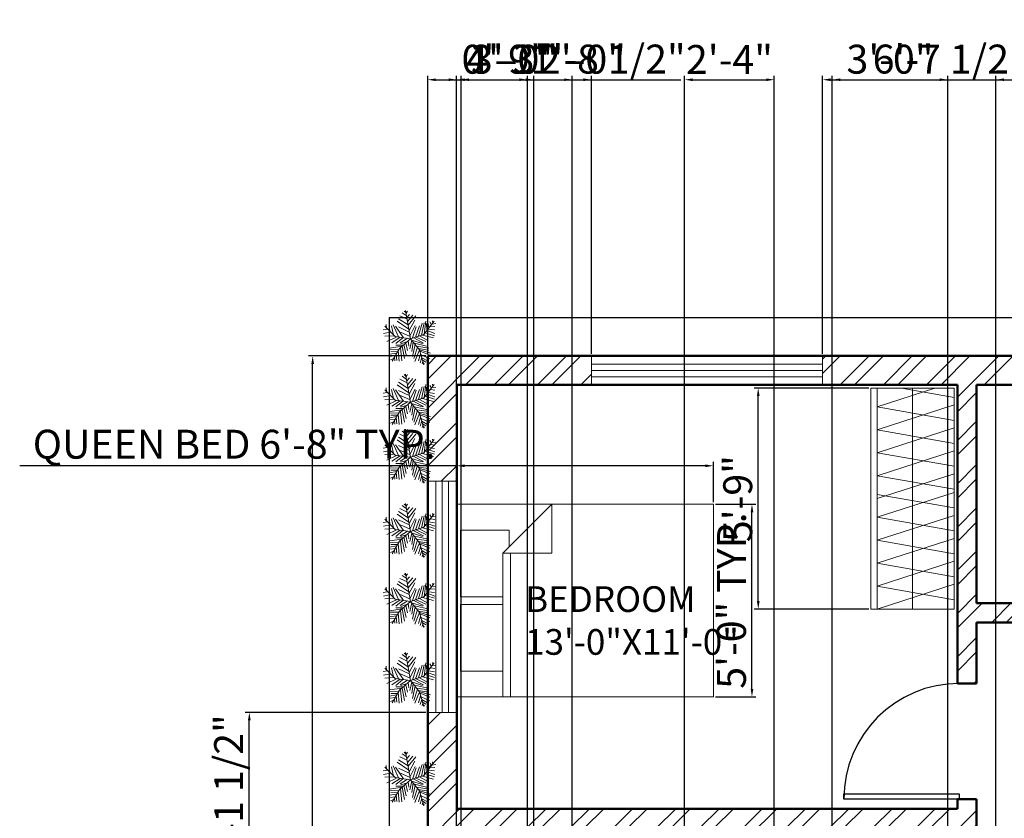
# Model space of a CAD drawing. Units: inches. Extents: x 176 to 806, y 915 to 1663.
# Tile 3 of 5: x 176 to 482, y 1414 to 1663. Entities that reach past the tile are written whole.
import ezdxf

# ---------------------------------------------------------------- set-up
doc = ezdxf.new("R2010")
doc.units = ezdxf.units.IN
for name, color, linetype, lineweight in [('A-ANNO-DIMS', 2, 'Continuous', 18), ('A-AREA-IDEN', 7, 'Continuous', 18), ('A-DOOR', 4, 'Continuous', 25), ('A-FLOR-CASE', 8, 'Continuous', 18), ('A-FURN', 8, 'Continuous', 18), ('A-WALL', 7, 'Continuous', 50), ('A-WALL-PATT', 252, 'Continuous', 13), ('C-PROP', 8, 'Continuous', 25), ('L-PLNT', 3, 'Continuous', 13)]:
    doc.layers.add(name, color=color, linetype=linetype, lineweight=lineweight)
doc.layers.add('A-GLAZ', color=244, linetype='Continuous', lineweight=18, true_color=0x991b1e)
doc.styles.get("Standard").update_dxf_attribs({"font": 'arial.ttf'})
doc.dimstyles.new('ISO-25', dxfattribs={"dimtxt": 9, "dimasz": 2.5, "dimexe": 1.25, "dimexo": 0.625, "dimtad": 1, "dimlunit": 3, "dimtxsty": 'Standard', "dimcen": 2.5, "dimadec": 0, "dimazin": 0, "dimtfac": 1, "dimtmove": 0, "dimatfit": 3, "dimfxl": 1, "dimarcsym": 0})

# ---------------------------------------------------------------- blocks, each defined once
blk = doc.blocks.new('*U4')
for p, q in [((-40, 0), (-40, 6)), ((0, 0), (0, 6))]:
    blk.add_line(p, q)
blk.add_lwpolyline([(0, 0), (0, -40), (-1.75, -40), (-1.75, 0)], close=True)
blk.add_arc((0, 0), 40, 180, 270)
blk = doc.blocks.new('*D10')
at = {"layer": 'A-ANNO-DIMS', "color": 0, "lineweight": -2, "transparency": 16777216}
for p, q in [((302.08, 1558.21), (265.58, 1558.21)), ((266.83, 1052.71), (266.83, 1555.71)), ((302.08, 1050.21), (265.58, 1050.21))]:
    blk.add_line(p, q, dxfattribs=at)
at = {"layer": 'A-ANNO-DIMS', "color": 0, "transparency": 16777216}
for points in [[(266.42, 1555.71), (267.25, 1555.71), (266.83, 1558.21)], [(266.42, 1052.71), (267.25, 1052.71), (266.83, 1050.21)]]:
    blk.add_solid(points, dxfattribs=at)
at = {"layer": 'Defpoints', "color": 0, "transparency": 16777216}
for p in [(266.83, 1558.21), (302.7, 1558.21), (302.7, 1050.21)]:
    blk.add_point(p, dxfattribs=at)
at = {"layer": 'A-ANNO-DIMS', "color": 0, "transparency": 16777216, "insert": (261.69, 1304.21), "char_height": 9, "attachment_point": 5, "rotation": 90}
blk.add_mtext('42\'-4"', dxfattribs=at)
blk = doc.blocks.new('Bed - Queen')
for p, q in [((0, -80.00003), (0, 0)), ((0, 0), (59.99999, 0)), ((59.99999, 0), (59.99999, -80.00003)), ((7.99999, -1.2), (28.79998, -1.2)), ((7.99999, -14.4), (7.99999, -1.2)), ((28.79998, -1.2), (28.79998, -14.4)), ((31.19999, -1.2), (51.99999, -1.2)), ((31.19999, -14.4), (31.19999, -1.2)), ((51.99999, -1.2), (51.99999, -16.4)), ((0, -14.4), (44.8, -14.4)), ((59.99999, -29.6), (44.8, -14.4)), ((44.8, -14.4), (44.8, -29.6)), ((44.8, -16.8), (0, -16.8)), ((51.99999, -16.4), (46.79936, -16.4)), ((44.8, -29.6), (59.99999, -29.6)), ((59.99999, -80.00003), (0, -80.00003))]:
    blk.add_line(p, q)
blk = doc.blocks.new('*U8')
for p, q in [((-5.114, 28.097), (-24.676, 40.636)), ((-7.288, 39.707), (-21.778, 46.673)), ((-8.737, 47.138), (-17.069, 52.711)), ((-10.186, 53.64), (-13.084, 55.962)), ((0, 0), (-10.5, 57)), ((-9.099, 51.782), (-6.563, 55.962)), ((-7.65, 43.423), (-2.578, 49.46)), ((-5.839, 35.992), (4.667, 48.067)), ((-5.114, 27.632), (10.463, 46.673)), ((-31.5, 4.5), (-52.5, 25.5)), ((-48.585, 21.131), (-49.309, 29.026)), ((-43.513, 28.561), (-42.427, 15.558)), ((-38.442, 26.239), (-34.819, 7.663)), ((-35.544, 28.097), (-24.314, 3.947)), ((-14.533, 2.09), (-30.834, 25.31)), ((-3.665, 19.273), (-27.574, 35.527)), ((-24.314, 23.917), (-2.941, 13.7)), ((-2.941, 16.486), (8.652, 37.85)), ((-1.129, 6.734), (9.014, 26.704)), ((3.942, 1.625), (11.187, 24.381)), ((10.101, 3.483), (17.708, 26.239)), ((16.259, 5.805), (23.142, 31.348)), ((22.055, 7.198), (27.489, 32.277)), ((27, 9), (48, 36)), ((27.127, 9.056), (31.112, 35.992)), ((31.836, 30.883), (32.561, 16.486)), ((35.096, 32.741), (37.27, 22.524)), ((38.719, 34.134), (41.979, 28.561)), ((40.53, 25.775), (48.862, 24.846)), ((43.791, 29.954), (51.036, 30.883)), ((44.153, 36.456), (45.239, 32.741)), ((-47.498, 19.737), (-55.83, 18.344)), ((-40.615, 13.7), (-55.105, 10.913)), ((-33.37, 6.269), (-52.207, 5.34)), ((-28.299, 3.483), (-47.86, -5.805)), ((-21.416, 3.018), (-38.079, -8.128)), ((0, 0), (-31.5, 4.5)), ((-15.982, 2.09), (-30.11, -9.521)), ((0, 0), (-22.5, -19.5)), ((-6.563, 1.161), (-21.416, -8.128)), ((-20.691, 13.7), (-1.129, 4.876)), ((0, 0), (27, 9)), ((0, 0), (18, -22.5)), ((6.478, 1.625), (26.04, -8.592)), ((11.187, 3.483), (30.749, -5.805)), ((18.07, 5.805), (35.096, -3.483)), ((24.229, 7.663), (46.688, 1.625)), ((29.662, 12.307), (48.137, 6.269)), ((33.285, 16.486), (48.862, 10.913)), ((36.183, 19.737), (48.137, 17.88)), ((-17.431, -15.094), (-42.789, -18.809)), ((-22.5, -19.5), (-37.5, -45)), ((-15.257, -12.772), (-30.11, -12.772)), ((-20.691, -18.345), (-17.793, -44.352)), ((-6.563, -5.805), (-19.967, -9.985)), ((-17.069, -15.094), (-12.721, -40.172)), ((-13.446, -11.378), (-8.737, -32.741)), ((-9.461, -8.592), (-6.201, -23.453)), ((-4.752, -3.483), (-3.665, -14.629)), ((2.493, -3.019), (-1.491, -20.202)), ((1.769, -2.555), (24.229, -9.521)), ((5.029, -6.27), (2.131, -25.775)), ((9.014, -11.378), (3.58, -35.992)), ((14.085, -16.951), (6.478, -40.172)), ((7.565, -9.056), (32.198, -14.629)), ((12.274, -15.094), (36.907, -18.809)), ((16.259, -19.738), (36.183, -22.989)), ((-28.299, -29.026), (-42.789, -31.348)), ((-24.314, -21.596), (-42.427, -22.06)), ((-30.834, -34.135), (-42.427, -35.528)), ((-34.457, -39.708), (-40.978, -42.494)), ((-26.849, -26.24), (-40.253, -25.775)), ((-32.646, -36.921), (-31.921, -44.352)), ((-29.023, -30.884), (-27.936, -43.887)), ((-25.038, -23.918), (-22.865, -45.281)), ((18.07, -22.524), (8.289, -45.745)), ((20.244, -30.419), (15.897, -44.816)), ((18, -22.5), (27, -52.5)), ((18.433, -22.524), (40.53, -29.026)), ((19.157, -25.311), (38.719, -33.206)), ((22.78, -37.85), (19.519, -48.532)), ((21.331, -32.741), (39.081, -40.636)), ((22.78, -38.314), (34.372, -44.816)), ((24.591, -45.745), (23.142, -50.854)), ((24.591, -43.423), (30.749, -47.603)), ((26.764, -49.925), (28.213, -50.854))]:
    blk.add_line(p, q)
blk = doc.blocks.new('WIN-GLAZING-72IN')
for p, q in [((0, 2), (72, 2)), ((0, 0), (72, 0)), ((0, -2), (72, -2))]:
    blk.add_line(p, q)
blk = doc.blocks.new('WARDROBE-HANGER')
for p, q in [((0, 0), (24, 7.76)), ((24, -4.24), (0, 0))]:
    blk.add_line(p, q)
blk = doc.blocks.new('*D28')
at = {"layer": 'A-ANNO-DIMS', "color": 0, "lineweight": -2, "transparency": 16777216}
for p, q in [((311.7, 1512.63), (311.7, 1525.26)), ((391.7, 1512.63), (391.7, 1525.26)), ((311.7, 1524.01), (175.56, 1524.01)), ((389.2, 1524.01), (314.2, 1524.01))]:
    blk.add_line(p, q, dxfattribs=at)
at = {"layer": 'A-ANNO-DIMS', "color": 0, "transparency": 16777216}
for points in [[(314.2, 1524.42), (314.2, 1523.59), (311.7, 1524.01)], [(389.2, 1524.42), (389.2, 1523.59), (391.7, 1524.01)]]:
    blk.add_solid(points, dxfattribs=at)
at = {"layer": 'Defpoints', "color": 0, "transparency": 16777216}
for p in [(311.7, 1524.01), (311.7, 1512.01), (391.7, 1512.01)]:
    blk.add_point(p, dxfattribs=at)
at = {"layer": 'A-ANNO-DIMS', "color": 0, "transparency": 16777216, "insert": (242.38, 1529.56), "char_height": 9, "attachment_point": 5}
blk.add_mtext('QUEEN BED 6\'-8" TYP.', dxfattribs=at)
blk = doc.blocks.new('*D29')
at = {"layer": 'A-ANNO-DIMS', "color": 0, "lineweight": -2, "transparency": 16777216}
for p, q in [((392.33, 1512.01), (404.95, 1512.01)), ((403.7, 1454.51), (403.7, 1509.51)), ((392.33, 1452.01), (404.95, 1452.01))]:
    blk.add_line(p, q, dxfattribs=at)
at = {"layer": 'A-ANNO-DIMS', "color": 0, "transparency": 16777216}
for points in [[(403.29, 1509.51), (404.12, 1509.51), (403.7, 1512.01)], [(403.29, 1454.51), (404.12, 1454.51), (403.7, 1452.01)]]:
    blk.add_solid(points, dxfattribs=at)
at = {"layer": 'Defpoints', "color": 0, "transparency": 16777216}
for p in [(391.7, 1512.01), (403.7, 1512.01), (391.7, 1452.01)]:
    blk.add_point(p, dxfattribs=at)
at = {"layer": 'A-ANNO-DIMS', "color": 0, "transparency": 16777216, "insert": (398.48, 1482.01), "char_height": 9, "attachment_point": 5, "rotation": 90}
blk.add_mtext('5\'-0" TYP.', dxfattribs=at)
blk = doc.blocks.new('*D40')
at = {"layer": 'A-ANNO-DIMS', "color": 0, "lineweight": -2, "transparency": 16777216}
for p, q in [((302.7, 1558.83), (302.7, 1645.51)), ((305.2, 1644.26), (351.2, 1644.26)), ((353.7, 1558.83), (353.7, 1645.51))]:
    blk.add_line(p, q, dxfattribs=at)
at = {"layer": 'A-ANNO-DIMS', "color": 0, "transparency": 16777216}
for points in [[(305.2, 1644.67), (305.2, 1643.84), (302.7, 1644.26)], [(351.2, 1644.67), (351.2, 1643.84), (353.7, 1644.26)]]:
    blk.add_solid(points, dxfattribs=at)
at = {"layer": 'Defpoints', "color": 0, "transparency": 16777216}
for p in [(353.7, 1644.26), (302.7, 1558.21), (353.7, 1558.21)]:
    blk.add_point(p, dxfattribs=at)
at = {"layer": 'A-ANNO-DIMS', "color": 0, "transparency": 16777216, "insert": (328.2, 1649.48), "char_height": 9, "attachment_point": 5}
blk.add_mtext('4\'-3"', dxfattribs=at)
blk = doc.blocks.new('*D41')
at = {"layer": 'A-ANNO-DIMS', "color": 0, "lineweight": -2, "transparency": 16777216}
for p, q in [((425.7, 1558.83), (425.7, 1645.51)), ((428.2, 1644.26), (502.7, 1644.26)), ((505.2, 1558.83), (505.2, 1645.51))]:
    blk.add_line(p, q, dxfattribs=at)
at = {"layer": 'A-ANNO-DIMS', "color": 0, "transparency": 16777216}
for points in [[(428.2, 1644.67), (428.2, 1643.84), (425.7, 1644.26)], [(502.7, 1644.67), (502.7, 1643.84), (505.2, 1644.26)]]:
    blk.add_solid(points, dxfattribs=at)
at = {"layer": 'Defpoints', "color": 0, "transparency": 16777216}
for p in [(505.2, 1644.26), (425.7, 1558.21), (505.2, 1558.21)]:
    blk.add_point(p, dxfattribs=at)
at = {"layer": 'A-ANNO-DIMS', "color": 0, "transparency": 16777216, "insert": (465.45, 1649.53), "char_height": 9, "attachment_point": 5}
blk.add_mtext('6\'-7 1/2"', dxfattribs=at)
blk = doc.blocks.new('*D48')
at = {"layer": 'A-ANNO-DIMS', "color": 0, "lineweight": -2, "transparency": 16777216}
for p, q in [((302.08, 1447.21), (245.85, 1447.21)), ((247.1, 1400.21), (247.1, 1444.71)), ((302.08, 1397.71), (245.85, 1397.71))]:
    blk.add_line(p, q, dxfattribs=at)
at = {"layer": 'A-ANNO-DIMS', "color": 0, "transparency": 16777216}
for points in [[(246.68, 1444.71), (247.52, 1444.71), (247.1, 1447.21)], [(246.68, 1400.21), (247.52, 1400.21), (247.1, 1397.71)]]:
    blk.add_solid(points, dxfattribs=at)
at = {"layer": 'Defpoints', "color": 0, "transparency": 16777216}
for p in [(247.1, 1447.21), (302.7, 1447.21), (302.7, 1397.71)]:
    blk.add_point(p, dxfattribs=at)
at = {"layer": 'A-ANNO-DIMS', "color": 0, "transparency": 16777216, "insert": (241.82, 1422.46), "char_height": 9, "attachment_point": 5, "rotation": 90}
blk.add_mtext('4\'-1 1/2"', dxfattribs=at)
blk = doc.blocks.new('*D50')
at = {"layer": 'A-ANNO-DIMS', "color": 0, "lineweight": -2, "transparency": 16777216}
for p, q in [((311.7, 1321.83), (311.7, 1645.51)), ((314.2, 1644.26), (345.2, 1644.26)), ((347.7, 1322.83), (347.7, 1645.51))]:
    blk.add_line(p, q, dxfattribs=at)
at = {"layer": 'A-ANNO-DIMS', "color": 0, "transparency": 16777216}
for points in [[(314.2, 1644.67), (314.2, 1643.84), (311.7, 1644.26)], [(345.2, 1644.67), (345.2, 1643.84), (347.7, 1644.26)]]:
    blk.add_solid(points, dxfattribs=at)
at = {"layer": 'Defpoints', "color": 0, "transparency": 16777216}
for p in [(347.7, 1644.26), (347.7, 1322.21), (311.7, 1321.21)]:
    blk.add_point(p, dxfattribs=at)
at = {"layer": 'A-ANNO-DIMS', "color": 0, "transparency": 16777216, "insert": (329.7, 1649.48), "char_height": 9, "attachment_point": 5}
blk.add_mtext('3\'-0"', dxfattribs=at)
blk = doc.blocks.new('*D52')
at = {"layer": 'A-ANNO-DIMS', "color": 0, "lineweight": -2, "transparency": 16777216}
for p, q in [((479.7, 1200.83), (479.7, 1645.51)), ((482.2, 1644.26), (525.2, 1644.26)), ((527.7, 1200.83), (527.7, 1645.51))]:
    blk.add_line(p, q, dxfattribs=at)
at = {"layer": 'A-ANNO-DIMS', "color": 0, "transparency": 16777216}
for points in [[(482.2, 1644.67), (482.2, 1643.84), (479.7, 1644.26)], [(525.2, 1644.67), (525.2, 1643.84), (527.7, 1644.26)]]:
    blk.add_solid(points, dxfattribs=at)
at = {"layer": 'Defpoints', "color": 0, "transparency": 16777216}
for p in [(527.7, 1644.26), (479.7, 1200.21), (527.7, 1200.21)]:
    blk.add_point(p, dxfattribs=at)
at = {"layer": 'A-ANNO-DIMS', "color": 0, "transparency": 16777216, "insert": (503.7, 1649.48), "char_height": 9, "attachment_point": 5}
blk.add_mtext('4\'-0"', dxfattribs=at)
blk = doc.blocks.new('*D53')
at = {"layer": 'A-ANNO-DIMS', "color": 0, "lineweight": -2, "transparency": 16777216}
for p, q in [((302.7, 1558.83), (302.7, 1645.51)), ((305.2, 1644.26), (309.2, 1644.26)), ((311.7, 1549.83), (311.7, 1645.51)), ((311.7, 1644.26), (339.38, 1644.26))]:
    blk.add_line(p, q, dxfattribs=at)
at = {"layer": 'A-ANNO-DIMS', "color": 0, "transparency": 16777216}
for points in [[(305.2, 1644.67), (305.2, 1643.84), (302.7, 1644.26)], [(309.2, 1644.67), (309.2, 1643.84), (311.7, 1644.26)]]:
    blk.add_solid(points, dxfattribs=at)
at = {"layer": 'Defpoints', "color": 0, "transparency": 16777216}
for p in [(311.7, 1644.26), (302.7, 1558.21), (311.7, 1549.21)]:
    blk.add_point(p, dxfattribs=at)
at = {"layer": 'A-ANNO-DIMS', "color": 0, "transparency": 16777216, "insert": (326.79, 1649.48), "char_height": 9, "attachment_point": 5}
blk.add_mtext('0\'-9"', dxfattribs=at)
blk = doc.blocks.new('*D57')
at = {"layer": 'A-ANNO-DIMS', "color": 0, "lineweight": -2, "transparency": 16777216}
for p, q in [((382.69, 1071.94), (382.69, 1645.51)), ((385.19, 1644.26), (408.14, 1644.26)), ((410.64, 1071.94), (410.64, 1645.51))]:
    blk.add_line(p, q, dxfattribs=at)
at = {"layer": 'A-ANNO-DIMS', "color": 0, "transparency": 16777216}
for points in [[(385.19, 1644.67), (385.19, 1643.84), (382.69, 1644.26)], [(408.14, 1644.67), (408.14, 1643.84), (410.64, 1644.26)]]:
    blk.add_solid(points, dxfattribs=at)
at = {"layer": 'Defpoints', "color": 0, "transparency": 16777216}
for p in [(410.64, 1644.26), (382.69, 1071.32), (410.64, 1071.32)]:
    blk.add_point(p, dxfattribs=at)
at = {"layer": 'A-ANNO-DIMS', "color": 0, "transparency": 16777216, "insert": (396.67, 1649.4), "char_height": 9, "attachment_point": 5}
blk.add_mtext('2\'-4"', dxfattribs=at)
blk = doc.blocks.new('*D59')
at = {"layer": 'A-ANNO-DIMS', "color": 0, "lineweight": -2, "transparency": 16777216}
for p, q in [((428.7, 1200.83), (428.7, 1645.51)), ((431.2, 1644.26), (462.2, 1644.26)), ((464.7, 1200.83), (464.7, 1645.51))]:
    blk.add_line(p, q, dxfattribs=at)
at = {"layer": 'A-ANNO-DIMS', "color": 0, "transparency": 16777216}
for points in [[(431.2, 1644.67), (431.2, 1643.84), (428.7, 1644.26)], [(462.2, 1644.67), (462.2, 1643.84), (464.7, 1644.26)]]:
    blk.add_solid(points, dxfattribs=at)
at = {"layer": 'Defpoints', "color": 0, "transparency": 16777216}
for p in [(464.7, 1644.26), (428.7, 1200.21), (464.7, 1200.21)]:
    blk.add_point(p, dxfattribs=at)
at = {"layer": 'A-ANNO-DIMS', "color": 0, "transparency": 16777216, "insert": (446.7, 1649.48), "char_height": 9, "attachment_point": 5}
blk.add_mtext('3\'-0"', dxfattribs=at)
blk = doc.blocks.new('*D61')
at = {"layer": 'A-ANNO-DIMS', "color": 0, "lineweight": -2, "transparency": 16777216}
for p, q in [((311.7, 1191.83), (311.7, 1645.51)), ((314.2, 1644.26), (333.2, 1644.26)), ((335.7, 1191.83), (335.7, 1645.51)), ((335.7, 1644.26), (363.53, 1644.26))]:
    blk.add_line(p, q, dxfattribs=at)
at = {"layer": 'A-ANNO-DIMS', "color": 0, "transparency": 16777216}
for points in [[(314.2, 1644.67), (314.2, 1643.84), (311.7, 1644.26)], [(333.2, 1644.67), (333.2, 1643.84), (335.7, 1644.26)]]:
    blk.add_solid(points, dxfattribs=at)
at = {"layer": 'Defpoints', "color": 0, "transparency": 16777216}
for p in [(335.7, 1644.26), (311.7, 1191.21), (335.7, 1191.21)]:
    blk.add_point(p, dxfattribs=at)
at = {"layer": 'A-ANNO-DIMS', "color": 0, "transparency": 16777216, "insert": (350.87, 1649.48), "char_height": 9, "attachment_point": 5}
blk.add_mtext('2\'-0"', dxfattribs=at)
blk = doc.blocks.new('*D62')
at = {"layer": 'A-ANNO-DIMS', "color": 0, "lineweight": -2, "transparency": 16777216}
for p, q in [((313.06, 1169.74), (313.06, 1645.51)), ((315.56, 1644.26), (331.24, 1644.26)), ((333.74, 1169.74), (333.74, 1645.51)), ((333.74, 1644.26), (381.54, 1644.26))]:
    blk.add_line(p, q, dxfattribs=at)
at = {"layer": 'A-ANNO-DIMS', "color": 0, "transparency": 16777216}
for points in [[(315.56, 1644.67), (315.56, 1643.84), (313.06, 1644.26)], [(331.24, 1644.67), (331.24, 1643.84), (333.74, 1644.26)]]:
    blk.add_solid(points, dxfattribs=at)
at = {"layer": 'Defpoints', "color": 0, "transparency": 16777216}
for p in [(333.74, 1644.26), (313.06, 1169.12), (333.74, 1169.12)]:
    blk.add_point(p, dxfattribs=at)
at = {"layer": 'A-ANNO-DIMS', "color": 0, "transparency": 16777216, "insert": (358.89, 1649.53), "char_height": 9, "attachment_point": 5}
blk.add_mtext('1\'-8 1/2"', dxfattribs=at)
blk = doc.blocks.new('*D69')
at = {"layer": 'A-ANNO-DIMS', "color": 0, "lineweight": -2, "transparency": 16777216}
for p, q in [((440.08, 1548.21), (404.4, 1548.21)), ((405.65, 1481.84), (405.65, 1545.71)), ((440.08, 1479.34), (404.4, 1479.34))]:
    blk.add_line(p, q, dxfattribs=at)
at = {"layer": 'A-ANNO-DIMS', "color": 0, "transparency": 16777216}
for points in [[(405.24, 1545.71), (406.07, 1545.71), (405.65, 1548.21)], [(405.24, 1481.84), (406.07, 1481.84), (405.65, 1479.34)]]:
    blk.add_solid(points, dxfattribs=at)
at = {"layer": 'Defpoints', "color": 0, "transparency": 16777216}
for p in [(405.65, 1548.21), (440.7, 1548.21), (440.7, 1479.34)]:
    blk.add_point(p, dxfattribs=at)
at = {"layer": 'A-ANNO-DIMS', "color": 0, "transparency": 16777216, "insert": (400.43, 1513.77), "char_height": 9, "attachment_point": 5, "rotation": 90}
blk.add_mtext('5\'-9"', dxfattribs=at)

msp = doc.modelspace()

# ---------------------------------------------------------------- hatches: boundary and pattern name
at = {"layer": 'A-WALL-PATT'}
h = msp.add_hatch(dxfattribs=at)
h.set_pattern_fill('ANSI32', color=256)
h.paths.add_polyline_path([(302.704, 1050.206), (353.704, 1050.206), (353.704, 1059.206), (311.704, 1059.206), (311.704, 1191.206), (428.704, 1191.206), (428.704, 1200.206), (311.704, 1200.206), (311.704, 1357.206), (473.704, 1357.206), (473.704, 1363.206), (408.704, 1363.206), (408.704, 1366.206), (402.704, 1366.206), (402.704, 1363.206), (311.704, 1363.206), (311.704, 1376.706), (302.704, 1376.706)])
h.paths.add_polyline_path([(311.704, 1447.206), (302.704, 1447.206), (302.704, 1397.706), (311.704, 1397.706), (311.704, 1411.206), (402.704, 1411.206), (402.704, 1396.206), (408.704, 1396.206), (408.704, 1411.206), (473.704, 1411.206), (473.704, 1420.206), (467.704, 1420.206), (467.704, 1417.206), (311.704, 1417.206)])
h.paths.add_polyline_path([(467.704, 1059.206), (425.704, 1059.206), (425.704, 1050.206), (476.704, 1050.206), (476.704, 1191.206), (479.704, 1191.206), (479.704, 1200.206), (464.704, 1200.206), (464.704, 1191.206), (467.704, 1191.206)])
h.paths.add_polyline_path([(719.704, 1278.206), (614.704, 1278.206), (614.704, 1272.206), (654.704, 1272.206), (654.704, 1250.311), (660.704, 1250.311), (660.704, 1272.206), (719.704, 1272.206), (719.704, 1246.706), (728.704, 1246.706), (728.704, 1307.669), (719.704, 1307.669)])
h.paths.add_polyline_path([(728.704, 1447.206), (719.704, 1447.206), (719.704, 1417.206), (563.704, 1417.206), (563.704, 1420.206), (557.704, 1420.206), (557.704, 1411.206), (569.704, 1411.206), (569.704, 1272.206), (578.704, 1272.206), (578.704, 1278.206), (575.704, 1278.206), (575.704, 1411.206), (719.704, 1411.206), (719.704, 1379.669), (728.704, 1379.669)])
h.paths.add_polyline_path([(677.704, 1558.206), (677.704, 1549.206), (719.704, 1549.206), (719.704, 1519.206), (728.704, 1519.206), (728.704, 1558.206)])
h.paths.add_polyline_path([(526.204, 1558.206), (526.204, 1549.206), (557.704, 1549.206), (557.704, 1481.206), (554.704, 1481.206), (554.704, 1475.206), (557.704, 1475.206), (557.704, 1456.206), (563.704, 1456.206), (563.704, 1549.206), (605.704, 1549.206), (605.704, 1558.206)])
h.paths.add_polyline_path([(425.704, 1558.206), (425.704, 1549.206), (467.704, 1549.206), (467.704, 1456.206), (473.704, 1456.206), (473.704, 1475.206), (524.704, 1475.206), (524.704, 1481.206), (473.704, 1481.206), (473.704, 1549.206), (505.204, 1549.206), (505.204, 1558.206)])
h.paths.add_polyline_path([(311.704, 1549.206), (353.704, 1549.206), (353.704, 1558.206), (302.704, 1558.206), (302.704, 1519.206), (311.704, 1519.206)])

# ---------------------------------------------------------------- linework, layer by layer
at = {"layer": 'A-FLOR-CASE'}
for p, q in [((440.704, 1548.206), (466.704, 1548.206)), ((440.704, 1548.206), (440.704, 1479.343)), ((442.704, 1548.206), (442.704, 1479.343)), ((442.704, 1542.391), (460.693, 1548.206)), ((466.704, 1545.309), (450.287, 1548.206)), ((453.704, 1548.206), (453.704, 1479.343)), ((466.704, 1548.206), (466.704, 1479.343)), ((466.704, 1538.155), (442.704, 1542.391)), ((442.704, 1513.775), (466.704, 1521.534)), ((466.704, 1510.878), (442.704, 1515.113)), ((442.704, 1479.343), (466.704, 1487.102)), ((440.704, 1479.343), (466.704, 1479.343))]:
    msp.add_line(p, q, dxfattribs=at)
at = {"layer": 'A-GLAZ'}
for points in [[(353.704, 1558.206), (425.704, 1558.206), (425.704, 1549.206), (353.704, 1549.206)], [(311.704, 1519.206), (311.704, 1447.206), (302.704, 1447.206), (302.704, 1519.206)]]:
    msp.add_lwpolyline(points, close=True, dxfattribs=at)
at = {"layer": 'A-WALL'}
for p, q in [((302.704, 1558.206), (302.704, 1050.206)), ((302.704, 1558.206), (728.704, 1558.206)), ((311.704, 1549.206), (467.704, 1549.206)), ((311.704, 1549.206), (311.704, 1417.206)), ((467.704, 1549.206), (467.704, 1456.206)), ((473.704, 1549.206), (473.704, 1481.206)), ((473.704, 1549.206), (557.704, 1549.206)), ((473.704, 1481.206), (524.704, 1481.206)), ((473.704, 1475.206), (524.704, 1475.206)), ((473.704, 1475.206), (473.704, 1456.206)), ((467.704, 1456.206), (473.704, 1456.206)), ((311.704, 1417.206), (467.704, 1417.206)), ((467.704, 1420.206), (473.704, 1420.206)), ((467.704, 1420.206), (467.704, 1417.206)), ((473.704, 1420.206), (473.704, 1411.206))]:
    msp.add_line(p, q, dxfattribs=at)
at = {"layer": 'C-PROP'}
for q in [(290.704, 1023.206), (740.704, 1570.206)]:
    msp.add_line((290.704, 1570.206), q, dxfattribs=at)

# ---------------------------------------------------------------- block references
at = {"layer": 'A-DOOR', "xscale": 0.9, "yscale": 0.9, "zscale": 0.9, "rotation": 269.9999999999985}
msp.add_blockref('*U4', (468.304, 1420.206), dxfattribs=at)
at = {"layer": 'A-FLOR-CASE'}
for p in [(442.704, 1535.237), (442.704, 1528.083), (442.704, 1520.929), (442.704, 1507.959), (442.704, 1500.805), (442.704, 1493.651), (442.704, 1486.497)]:
    msp.add_blockref('WARDROBE-HANGER', p, dxfattribs=at)
at = {"layer": 'A-FURN', "rotation": 90}
msp.add_blockref('Bed - Queen', (311.704, 1452.006), dxfattribs=at)
at = {"layer": 'A-GLAZ'}
msp.add_blockref('WIN-GLAZING-72IN', (353.704, 1553.706), dxfattribs=at)
at = {"layer": 'A-GLAZ', "rotation": 89.99999999999991}
msp.add_blockref('WIN-GLAZING-72IN', (307.204, 1447.206), dxfattribs=at)
at = {"layer": 'L-PLNT', "xscale": 0.1538165911341002, "yscale": 0.1538165911341002, "zscale": 0.1538165911341002}
for p in [(297.354, 1563.563), (297.354, 1543.785), (297.354, 1526.653), (297.354, 1503.49), (297.354, 1481.763), (297.354, 1457.081), (297.354, 1426.191)]:
    msp.add_blockref('*U8', p, dxfattribs=at)

# ---------------------------------------------------------------- texts
at = {"layer": 'A-AREA-IDEN', "insert": (333.024, 1486.48), "char_height": 8, "attachment_point": 1}
msp.add_mtext_dynamic_manual_height_columns('BEDROOM\\P13\'-0"X11\'-0"', width=67.48766, gutter_width=12.5, heights=[0], dxfattribs=at)

# ---------------------------------------------------------------- dimensions: what is measured, and where the dimension line sits
at = {"layer": 'A-ANNO-DIMS'}
for base, p1, p2, picture, middle in [((333.742, 1644.256), (313.064, 1169.115), (333.742, 1169.115), '*D62', (358.892, 1649.535)), ((505.204, 1644.256), (425.704, 1558.206), (505.204, 1558.206), '*D41', (465.454, 1649.535)), ((353.704, 1644.256), (302.704, 1558.206), (353.704, 1558.206), '*D40', (328.204, 1649.48)), ((311.704, 1644.256), (302.704, 1558.206), (311.704, 1549.206), '*D53', (326.791, 1649.477)), ((347.704, 1644.256), (311.704, 1321.206), (347.704, 1322.206), '*D50', (329.704, 1649.48)), ((335.704, 1644.256), (311.704, 1191.206), (335.704, 1191.206), '*D61', (350.868, 1649.477)), ((410.644, 1644.256), (382.695, 1071.316), (410.644, 1071.316), '*D57', (396.669, 1649.4)), ((464.704, 1644.256), (428.704, 1200.206), (464.704, 1200.206), '*D59', (446.704, 1649.48)), ((527.704, 1644.256), (479.704, 1200.206), (527.704, 1200.206), '*D52', (503.704, 1649.477))]:
    dim = msp.add_linear_dim(base=base, p1=p1, p2=p2, dimstyle='ISO-25', override={"dimdec": 1, "dimlfac": 1, "dimrnd": 0, "dimzin": 1, "dimdsep": 46, "dimlunit": 4, "dimfrac": 2}, dxfattribs=at)
    dim.commit()
    dim.dimension.update_dxf_attribs({"geometry": picture, "text_midpoint": middle})
for base, p1, p2, angle, text, picture, middle in [((311.704, 1524.006), (391.704, 1512.006), (311.704, 1512.006), 180, 'QUEEN BED <> TYP.', '*D28', (242.383, 1529.561)), ((403.704, 1512.006), (391.704, 1452.006), (391.704, 1512.006), 90, '<> TYP.', '*D29', (398.484, 1482.006))]:
    dim = msp.add_linear_dim(base=base, p1=p1, p2=p2, angle=angle, text=text, dimstyle='ISO-25', override={"dimdec": 1, "dimlfac": 1, "dimrnd": 0, "dimzin": 1, "dimdsep": 46, "dimlunit": 4, "dimfrac": 2}, dxfattribs=at)
    dim.commit()
    dim.dimension.update_dxf_attribs({"geometry": picture, "text_midpoint": middle})
for base, p1, p2, override, picture, middle in [((266.833, 1558.206), (302.704, 1050.206), (302.704, 1558.206), {"dimclrd": 0, "dimclre": 0, "dimclrt": 0}, '*D10', (261.689, 1304.206)), ((405.654, 1548.206), (440.704, 1479.343), (440.704, 1548.206), {"dimdec": 1, "dimlfac": 1, "dimrnd": 0, "dimzin": 1, "dimdsep": 46, "dimlunit": 4, "dimfrac": 2}, '*D69', (400.434, 1513.775)), ((247.1, 1447.206), (302.704, 1397.706), (302.704, 1447.206), {"dimdec": 1, "dimlfac": 1, "dimrnd": 0, "dimzin": 1, "dimdsep": 46, "dimlunit": 4, "dimfrac": 2}, '*D48', (241.821, 1422.456))]:
    dim = msp.add_linear_dim(base=base, p1=p1, p2=p2, angle=90, dimstyle='ISO-25', override=override, dxfattribs=at)
    dim.commit()
    dim.dimension.update_dxf_attribs({"geometry": picture, "text_midpoint": middle})

doc.saveas('drawing.dxf')
